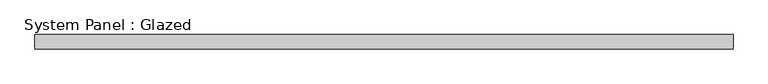
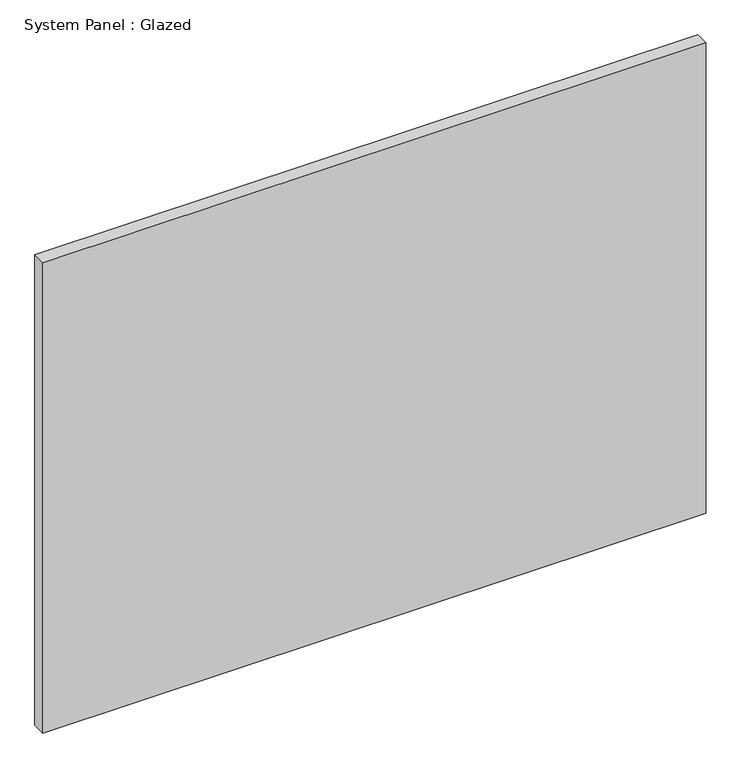
"""IFC4 building model written with IfcOpenShell, lengths in millimetres: plate geometry, System Panel : Glazed."""

from ifc_helpers import new_model, si_unit, origin, origin_with_axes, place, context, project, spatial, polyline, outline, extrude, source, transform, mapped, element, save


def system_panel_glazed_cfef7f4a(model_context):
    return source(origin(), model_context, "Body", "SweptSolid", [
        extrude(outline(polyline([(609.6680043, 19.05), (-609.6680043, 19.05), (-609.6680043, 44.45), (609.6680043, 44.45), (609.6680043, 19.05)])), origin_with_axes(), (0.0, 0.0, 1.0), 914.4),
    ])


if __name__ == "__main__":
    model = new_model("IFC4")
    model_context = context("Model", 3, world=origin())
    ifc_project = project(units=[si_unit("LENGTHUNIT", "METRE", prefix="MILLI")], contexts=[model_context])
    site = spatial("IfcSite", under=ifc_project)
    building = spatial("IfcBuilding", under=site)
    placement = place(None, origin())
    system_panel_glazed_shape = system_panel_glazed_cfef7f4a(model_context)
    element("IfcPlate", 1, ObjectType="System Panel : Glazed", at=placement, inside=building, context=model_context, shape_type="MappedRepresentation", body=[
        mapped(system_panel_glazed_shape, transform((0.0, 0.0, 0.0), x_axis=(1.0, 0.0, 0.0), y_axis=(0.0, 1.0, 0.0), z_axis=(0.0, 0.0, 1.0))),
    ])
    save(model, "model.ifc")

# Revit data of these elements
# Type "System Panel : Glazed"
#   Construction Type Id = "GSP4R"
#   Analytic Construction = "1/8 in Pilkington single glazing"
#   Visual Light Transmittance = 0.9
#   Solar Heat Gain Coefficient = 0.86
#   Heat Transfer Coefficient (U) = 1.18115 BTU/(h·ft²·°F)
# Element 1 (IfcPlate, "System Panel : Glazed")
#   Materials on its faces: "Glass"
# Materials
#   "Glass": class "Glass", colour RGB 0 128 192, transparency 0.75, Description = "Soda Lime Glass", Cost = 0
